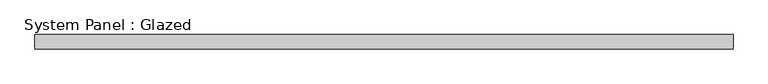
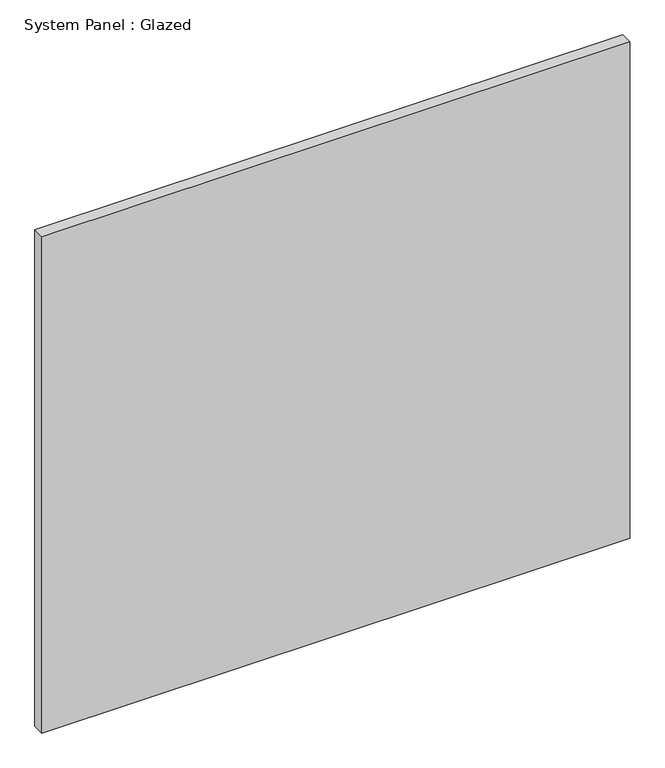
"""IFC4 building model written with IfcOpenShell, lengths in millimetres: plate geometry, System Panel : Glazed."""

from ifc_helpers import new_model, si_unit, origin, origin_with_axes, place, context, project, spatial, polyline, outline, extrude, source, transform, mapped, element, save


def system_panel_glazed_c8a97ecb(model_context):
    return source(origin(), model_context, "Body", "SweptSolid", [
        extrude(outline(polyline([(611.3440639, 19.05), (-611.3440639, 19.05), (-611.3440639, 44.45), (611.3440639, 44.45), (611.3440639, 19.05)])), origin_with_axes(), (0.0, 0.0, 1.0), 1092.2),
    ])


if __name__ == "__main__":
    model = new_model("IFC4")
    model_context = context("Model", 3, world=origin())
    ifc_project = project(units=[si_unit("LENGTHUNIT", "METRE", prefix="MILLI")], contexts=[model_context])
    site = spatial("IfcSite", under=ifc_project)
    building = spatial("IfcBuilding", under=site)
    placement = place(None, origin())
    system_panel_glazed_shape = system_panel_glazed_c8a97ecb(model_context)
    element("IfcPlate", 1, ObjectType="System Panel : Glazed", at=placement, inside=building, context=model_context, shape_type="MappedRepresentation", body=[
        mapped(system_panel_glazed_shape, transform((0.0, 0.0, 0.0), x_axis=(1.0, 0.0, 0.0), y_axis=(0.0, 1.0, 0.0), z_axis=(0.0, 0.0, 1.0))),
    ])
    save(model, "model.ifc")

# Revit data of these elements
# Type "System Panel : Glazed"
#   Construction Type Id = "GSP4R"
#   Analytic Construction = "1/8 in Pilkington single glazing"
#   Visual Light Transmittance = 0.9
#   Solar Heat Gain Coefficient = 0.86
#   Heat Transfer Coefficient (U) = 1.18115 BTU/(h·ft²·°F)
#   Define Thermal Properties by = 1
# Element 1 (IfcPlate, "System Panel : Glazed")
#   Materials on its faces: "Glass"
# Materials
#   "Glass": class "Glass", colour RGB 0 128 192, transparency 0.75, Description = "Soda Lime Glass", Cost = 0
